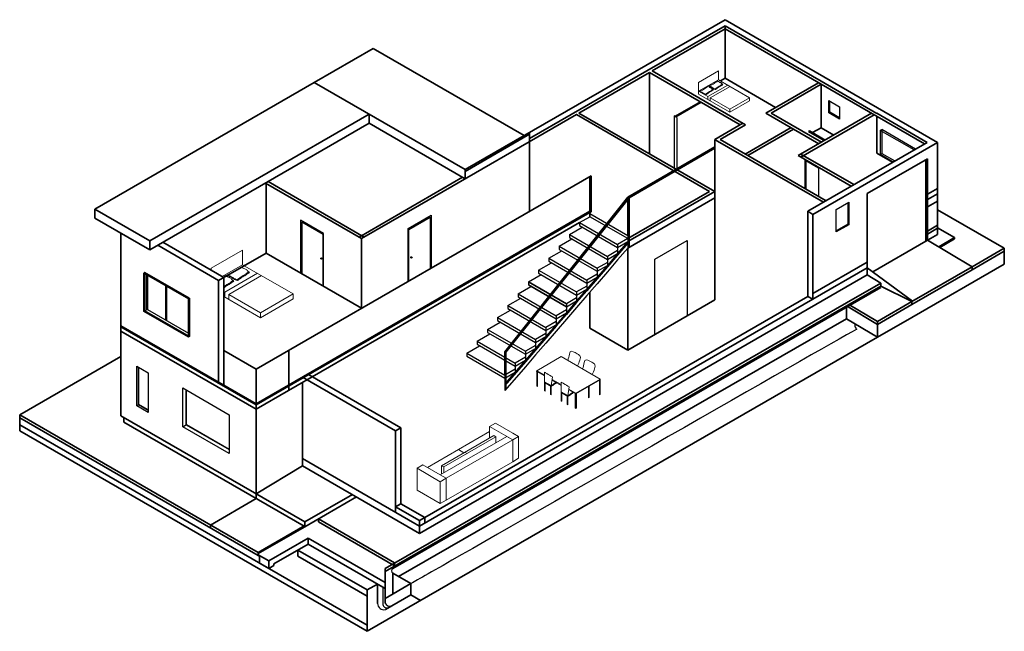
# Model space of a CAD drawing. Units: millimetres. Extents: x -3210 to 34050, y 6347 to 29494.
import ezdxf

# ---------------------------------------------------------------- set-up
doc = ezdxf.new("R2010")
doc.units = ezdxf.units.MM
for name, color, linetype, lineweight in [('A-DOOR', 4, 'Continuous', 25), ('A-FLOR-FIXT', 8, 'Continuous', 18), ('A-FLOR-STRS', 2, 'Continuous', 25), ('A-FURN', 8, 'Continuous', 18), ('A-GLAZ', 3, 'Continuous', 25), ('A-WALL', 7, 'Continuous', 35), ('C-STRM', 5, 'Continuous', 25)]:
    doc.layers.add(name, color=color, linetype=linetype, lineweight=lineweight)

# ---------------------------------------------------------------- blocks, each defined once
blk = doc.blocks.new('stairs')
for p, q in [((17980, 21815), (18368, 22039)), ((19805, 21320), (18368, 22153)), ((19805, 21209), (18368, 22039)), ((17592, 21366), (18076, 21645)), ((17980, 21815), (19417, 20985)), ((17980, 21815), (17980, 21701)), ((17980, 21701), (19417, 20871)), ((17592, 21366), (19029, 20536)), ((17592, 21366), (17592, 21252)), ((17592, 21252), (19029, 20422)), ((19805, 21320), (19805, 20849)), ((17204, 20917), (17688, 21196)), ((17204, 20917), (18641, 20087)), ((17204, 20917), (17204, 20803)), ((19805, 21209), (19417, 20985)), ((19417, 20871), (19805, 21095)), ((19417, 20985), (19417, 20871)), ((19417, 20871), (19417, 20646)), ((16816, 20468), (17300, 20747)), ((17204, 20803), (18641, 19973)), ((19417, 20760), (19029, 20536)), ((19029, 20422), (19417, 20646)), ((19029, 20536), (19029, 20422)), ((16428, 20019), (16912, 20298)), ((16816, 20468), (18253, 19638)), ((16816, 20468), (16816, 20354)), ((16816, 20354), (18253, 19524)), ((19029, 20311), (18641, 20087)), ((18641, 19973), (19029, 20197)), ((19029, 20422), (19029, 20197)), ((16040, 19570), (16524, 19849)), ((16428, 20019), (17865, 19189)), ((16428, 20019), (16428, 19905)), ((16428, 19905), (17865, 19075)), ((18641, 19862), (18253, 19638)), ((18253, 19524), (18641, 19748)), ((18641, 20087), (18641, 19973)), ((18641, 19973), (18641, 19748)), ((15652, 19121), (16136, 19400)), ((16040, 19570), (16040, 19456)), ((18253, 19413), (17865, 19189)), ((18253, 19638), (18253, 19524)), ((18253, 19524), (18253, 19299)), ((15652, 19121), (17089, 18291)), ((15652, 19121), (15652, 19007)), ((15652, 19007), (17089, 18177)), ((17865, 19075), (18253, 19299)), ((17865, 19189), (17865, 19075)), ((17865, 19075), (17865, 18850)), ((15264, 18672), (15748, 18951)), ((15264, 18672), (16701, 17842)), ((15264, 18672), (15264, 18558)), ((17865, 18964), (17477, 18740)), ((17477, 18626), (17865, 18850)), ((17477, 18740), (17477, 18626)), ((14876, 18223), (15360, 18502)), ((15264, 18558), (16701, 17728)), ((17477, 18515), (17089, 18291)), ((17089, 18177), (17477, 18401)), ((17089, 18291), (17089, 18177)), ((17477, 18626), (17477, 18401)), ((14488, 17774), (14972, 18053)), ((14876, 18223), (16314, 17393)), ((14876, 18223), (14876, 18109)), ((14876, 18109), (16314, 17279)), ((17089, 18066), (16701, 17842)), ((16701, 17728), (17089, 17952)), ((17089, 18177), (17089, 17952)), ((14100, 17325), (14584, 17604)), ((14488, 17774), (15926, 16944)), ((14488, 17774), (14488, 17660)), ((14488, 17660), (15926, 16830)), ((16701, 17617), (16314, 17393)), ((16701, 17842), (16701, 17728)), ((16701, 17728), (16701, 17503)), ((13712, 16876), (14196, 17155)), ((14100, 17325), (15538, 16495)), ((14100, 17325), (14100, 17211)), ((14100, 17211), (15538, 16381)), ((16314, 17168), (15926, 16944)), ((16314, 17279), (16701, 17503)), ((16314, 17393), (16314, 17279)), ((16314, 17279), (16314, 17054)), ((13712, 16876), (15150, 16046)), ((13712, 16876), (13712, 16762)), ((15926, 16830), (16314, 17054)), ((15926, 16944), (15926, 16830)), ((15926, 16830), (15926, 16605)), ((13712, 16762), (15150, 15932)), ((15926, 16719), (15538, 16495)), ((15538, 16381), (15926, 16605)), ((15538, 16495), (15538, 16381)), ((15538, 16270), (15150, 16046)), ((15150, 15932), (15538, 16156)), ((15150, 16046), (15150, 15932)), ((15538, 16381), (15538, 16156)), ((15150, 15932), (15150, 15461))]:
    blk.add_line(p, q)
for points in [[(19805, 21095), (19417, 20646), (19029, 20197), (18641, 19748), (18253, 19299), (17865, 18850), (17477, 18401), (17089, 17952), (16701, 17503), (16314, 17054), (15926, 16605), (15150, 15707)], [(19805, 21033), (19417, 20584), (19029, 20135), (18641, 19686), (18253, 19237), (17865, 18788), (17477, 18339), (17089, 17890), (16701, 17441), (16314, 16992), (15926, 16543), (15150, 15645)], [(19805, 20849), (19417, 20400), (19029, 19951), (18641, 19502), (18253, 19053), (17865, 18604), (17477, 18155), (17089, 17706), (16701, 17257), (16314, 16808), (15926, 16359), (15150, 15461)]]:
    blk.add_lwpolyline(points)
blk = doc.blocks.new('dininig')
for p, q in [((17285, 16742), (16365, 16211)), ((18753, 15894), (17285, 16742)), ((16365, 16211), (16646, 16049)), ((16365, 16211), (16365, 15625)), ((16365, 16178), (16646, 16016)), ((16387, 15612), (16387, 16166)), ((16646, 15793), (16646, 15447)), ((16646, 15793), (16900, 15646)), ((16646, 15759), (16900, 15612)), ((16669, 15745), (16669, 15433)), ((16932, 15851), (17281, 15649)), ((16937, 15881), (17281, 15682)), ((17834, 15363), (18753, 15894)), ((17834, 15331), (18753, 15861)), ((18731, 15295), (18731, 15849)), ((18753, 15894), (18753, 15861)), ((18753, 15861), (18753, 15308)), ((16365, 15625), (16387, 15612)), ((16669, 15433), (16646, 15447)), ((16877, 15625), (16877, 15313)), ((16877, 15313), (16900, 15300)), ((16900, 15646), (16900, 15300)), ((17281, 15414), (17281, 15068)), ((17281, 15414), (17536, 15267)), ((17281, 15380), (17536, 15233)), ((17304, 15367), (17304, 15054)), ((17569, 15483), (17834, 15331)), ((17574, 15513), (17834, 15363)), ((17812, 14789), (17812, 15343)), ((17834, 15331), (17834, 14777)), ((17855, 14789), (17855, 15343)), ((18318, 15186), (18318, 15611)), ((18340, 15623), (18340, 15199)), ((18753, 15308), (18731, 15295)), ((17513, 15246), (17513, 14934)), ((17513, 14934), (17536, 14921)), ((17536, 15267), (17536, 14921)), ((18340, 15199), (18318, 15186)), ((17834, 14777), (17812, 14789)), ((17834, 14777), (17855, 14789))]:
    blk.add_line(p, q)
for centre in [(17067, 15749), (17703, 15370)]:
    blk.add_arc(centre, 20.9, 300.0624, 62.4998)
for points, knots in [([(17535, 16602), (17556, 16677), (17584, 16778), (17623, 17007), (17844, 16872), (18083, 16748), (17948, 16515), (17902, 16387), (17901, 16386)], [0, 0, 0, 0, 244.890523, 329.00144, 608.473459, 721.036072, 1125.699972, 1130.16971, 1130.16971, 1130.16971, 1130.16971]), ([(18091, 16281), (18113, 16356), (18141, 16457), (18180, 16685), (18401, 16551), (18639, 16427), (18505, 16193), (18458, 16066), (18458, 16064)], [0, 0, 0, 0, 244.890523, 329.00144, 608.473459, 721.036072, 1125.699972, 1130.16971, 1130.16971, 1130.16971, 1130.16971]), ([(16646, 16154), (16676, 16136), (16778, 16077), (16880, 16018), (16952, 15977)], [0, 0, 0, 0, 105.813735, 353.485059, 353.485059, 353.485059, 353.485059]), ([(16900, 15612), (16921, 15626), (16983, 15668), (17044, 15709), (17078, 15731)], [0, 0, 0, 0, 75.861008, 223.095154, 223.095154, 223.095154, 223.095154]), ([(17281, 15775), (17312, 15757), (17414, 15698), (17516, 15639), (17587, 15598)], [0, 0, 0, 0, 105.813735, 353.485059, 353.485059, 353.485059, 353.485059]), ([(17536, 15233), (17557, 15247), (17618, 15289), (17680, 15330), (17713, 15352)], [0, 0, 0, 0, 75.861008, 223.095154, 223.095154, 223.095154, 223.095154])]:
    blk.add_open_spline(points, degree=3, knots=knots)
for points in [[(16646, 15793), (16646, 15913), (16646, 16033), (16646, 16154)], [(16900, 15646), (16917, 15756), (16934, 15867), (16952, 15977)], [(16900, 15646), (16959, 15686), (17018, 15727), (17077, 15767)], [(17281, 15414), (17281, 15534), (17281, 15655), (17281, 15775)], [(17536, 15267), (17553, 15377), (17570, 15488), (17587, 15598)], [(17536, 15267), (17595, 15308), (17654, 15348), (17713, 15389)]]:
    blk.add_open_spline(points, degree=3)
blk = doc.blocks.new('sofa')
for p, q in [((14566, 14099), (14789, 14228)), ((14789, 14228), (15446, 13849)), ((12217, 12549), (14566, 13905)), ((15446, 13591), (14566, 14099)), ((14566, 14099), (14566, 13658)), ((15669, 13720), (15446, 13849)), ((12705, 12267), (15222, 13720)), ((12758, 12614), (14730, 13753)), ((12838, 12568), (14810, 13706)), ((12929, 12138), (15446, 13591)), ((14730, 13753), (14810, 13706)), ((14810, 13706), (14810, 13482)), ((15222, 13720), (15446, 13591)), ((15669, 13720), (15446, 13591)), ((15446, 13591), (15446, 12765)), ((15446, 12765), (15446, 13591)), ((15669, 12894), (15669, 13720)), ((13391, 13227), (13601, 13101)), ((13637, 13122), (13717, 13076)), ((12929, 11312), (15446, 12765)), ((15669, 12894), (15446, 12765)), ((11825, 12517), (12049, 12646)), ((12705, 12009), (11825, 12517)), ((11825, 12517), (11825, 11691)), ((12049, 12646), (12705, 12267)), ((12758, 12297), (12758, 12614)), ((12758, 12614), (12838, 12568)), ((12838, 12343), (12838, 12568)), ((12929, 12138), (12705, 12267)), ((12929, 12138), (12705, 12009)), ((12705, 11183), (12705, 12009)), ((12929, 11312), (12929, 12138)), ((12705, 11183), (11825, 11691)), ((12929, 11312), (12705, 11183))]:
    blk.add_line(p, q)
blk = doc.blocks.new('DOOR-900')
for p, q in [((0, 2000), (866, 2500)), ((17, 1960), (823, 2425)), ((823, 2425), (823, 475)), ((866, 2500), (866, 500)), ((0, 0), (0, 2000)), ((17, 10), (17, 1960))]:
    blk.add_line(p, q)
blk = doc.blocks.new('SINK-BOWL')
for p, q in [((0, 134), (4, 114)), ((503, 200), (507, 180))]:
    blk.add_line(p, q)
blk.add_arc((252, 15), 27.2, 169.8269, 214.4645)
for points, knots in [([(0, 134), (17, 144), (48, 164), (141, 193), (223, 262), (299, 304), (323, 317)], [0, 0, 0, 0, 58.087892, 110.763148, 288.499212, 372.227316, 372.227316, 372.227316, 372.227316]), ([(0, 134), (35, 118), (95, 90), (165, 42), (208, 26), (225, 20)], [0, 0, 0, 0, 115.602535, 198.179559, 253.050311, 253.050311, 253.050311, 253.050311]), ([(4, 114), (39, 98), (99, 70), (169, 21), (212, 6), (230, 0)], [0, 0, 0, 0, 115.602535, 198.179559, 253.050311, 253.050311, 253.050311, 253.050311]), ([(225, 20), (250, 38), (298, 73), (355, 118), (422, 143), (427, 163), (474, 187), (475, 189), (476, 191), (485, 194), (494, 197), (503, 200)], [0, 0, 0, 0, 88.806256, 177.702848, 228.702299, 271.942722, 280.573254, 305.589533, 305.589533, 305.589533, 331.140258, 331.140258, 331.140258, 331.140258]), ([(230, 0), (254, 17), (303, 52), (359, 98), (426, 123), (432, 143), (478, 167), (479, 169), (480, 171), (489, 174), (498, 177), (507, 180)], [0, 0, 0, 0, 88.806256, 177.702848, 228.702299, 271.942722, 280.573254, 305.589533, 305.589533, 305.589533, 331.140258, 331.140258, 331.140258, 331.140258]), ([(323, 317), (342, 304), (373, 283), (415, 265), (451, 255), (460, 225), (476, 216), (483, 212), (490, 208), (496, 204), (503, 200)], [0, 0, 0, 0, 68.223474, 110.975196, 140.481146, 170.504076, 194.596577, 194.596577, 194.596577, 217.431117, 217.431117, 217.431117, 217.431117])]:
    blk.add_open_spline(points, degree=3, knots=knots)

msp = doc.modelspace()

# ---------------------------------------------------------------- linework, layer by layer
at = {"layer": 'A-DOOR'}
for p, q in [((21551, 25852), (21551, 23884)), ((21653, 25793), (21551, 25852)), ((21653, 25793), (21653, 23825)), ((26501, 24208), (26501, 23108)), ((26540, 24166), (27012, 23893)), ((26540, 24166), (26540, 23086)), ((27012, 23893), (27012, 22813)), ((27020, 23908), (27020, 22808)), ((20824, 20429), (22052, 21138)), ((22052, 21138), (22052, 18287)), ((20824, 17578), (20824, 20429))]:
    msp.add_line(p, q, dxfattribs=at)
for centre, radius in [((11613, 20495), 26.5), ((8205, 20457), 23.3)]:
    msp.add_circle(centre, radius, dxfattribs=at)
at = {"layer": 'A-FLOR-FIXT'}
for p, q in [((22477, 27122), (23234, 27559)), ((22477, 26786), (23234, 27222)), ((23234, 27222), (23234, 27559)), ((23234, 27222), (24413, 26542)), ((22477, 26786), (22477, 27122)), ((22825, 26585), (23582, 27022)), ((22918, 26531), (23674, 26968)), ((22477, 26786), (22477, 26670)), ((22825, 26585), (22477, 26786)), ((23657, 25990), (22477, 26670)), ((22825, 26585), (22825, 26470)), ((23657, 26105), (22918, 26531)), ((22918, 26531), (22918, 26416)), ((24413, 26542), (23657, 26105)), ((24413, 26542), (24413, 26426)), ((24413, 26426), (23657, 25990)), ((23657, 26105), (23657, 25990)), ((4040, 20090), (5219, 20770)), ((5219, 20223), (5219, 20770)), ((4448, 19778), (5219, 20223)), ((5219, 20223), (7139, 19115)), ((4040, 20013), (4040, 20090)), ((4553, 19186), (5785, 19897)), ((4654, 19838), (4661, 19805)), ((4705, 19098), (5936, 19809)), ((5473, 19945), (5480, 19912)), ((4882, 19617), (4889, 19584)), ((4553, 19186), (4515, 19208)), ((5907, 18217), (4515, 19021)), ((4553, 19186), (4553, 18998)), ((5907, 18404), (4705, 19098)), ((4705, 19098), (4705, 18911)), ((7139, 19115), (5907, 18404)), ((7139, 19115), (7139, 18928)), ((7139, 18928), (5907, 18217)), ((5907, 18404), (5907, 18217))]:
    msp.add_line(p, q, dxfattribs=at)
msp.add_arc((5064, 19645), 44.3, 169.8269, 214.4645, dxfattribs=at)
for points, knots in [([(4654, 19838), (4681, 19855), (4733, 19886), (4883, 19933), (5016, 20046), (5141, 20114), (5180, 20136)], [0, 0, 0, 0, 94.538199, 180.267318, 469.533235, 605.800947, 605.800947, 605.800947, 605.800947]), ([(5180, 20136), (5211, 20114), (5261, 20079), (5330, 20051), (5387, 20034), (5402, 19986), (5428, 19971), (5440, 19964), (5451, 19958), (5462, 19951), (5473, 19945)], [0, 0, 0, 0, 68.223474, 110.975196, 140.481146, 170.504076, 194.596577, 194.596577, 194.596577, 217.431117, 217.431117, 217.431117, 217.431117]), ([(4590, 19808), (4620, 19786), (4670, 19751), (4739, 19723), (4797, 19706), (4811, 19658), (4837, 19643), (4849, 19636), (4860, 19630), (4871, 19623), (4882, 19617)], [0, 0, 0, 0, 68.223474, 110.975196, 140.481146, 170.504076, 194.596577, 194.596577, 194.596577, 217.431117, 217.431117, 217.431117, 217.431117]), ([(4654, 19838), (4711, 19812), (4809, 19767), (4922, 19687), (4993, 19662), (5021, 19652)], [0, 0, 0, 0, 188.143434, 322.53776, 411.840053, 411.840053, 411.840053, 411.840053]), ([(4661, 19805), (4718, 19779), (4816, 19734), (4929, 19654), (5000, 19629), (5028, 19619)], [0, 0, 0, 0, 188.143434, 322.53776, 411.840053, 411.840053, 411.840053, 411.840053]), ([(5021, 19652), (5060, 19681), (5139, 19738), (5231, 19812), (5341, 19853), (5349, 19884), (5425, 19923), (5427, 19927), (5429, 19930), (5443, 19935), (5458, 19940), (5473, 19945)], [0, 0, 0, 0, 88.806256, 177.702848, 228.702299, 271.942722, 280.573254, 305.589533, 305.589533, 305.589533, 331.140258, 331.140258, 331.140258, 331.140258]), ([(5028, 19619), (5067, 19648), (5146, 19705), (5238, 19779), (5348, 19820), (5357, 19852), (5432, 19891), (5434, 19894), (5436, 19897), (5451, 19902), (5465, 19907), (5480, 19912)], [0, 0, 0, 0, 88.806256, 177.702848, 228.702299, 271.942722, 280.573254, 305.589533, 305.589533, 305.589533, 331.140258, 331.140258, 331.140258, 331.140258]), ([(4515, 19386), (4525, 19394), (4574, 19430), (4641, 19483), (4750, 19525), (4759, 19556), (4835, 19595), (4837, 19599), (4838, 19602), (4853, 19607), (4867, 19612), (4882, 19617)], [63.928623, 63.928623, 63.928623, 63.928623, 88.806256, 177.702848, 228.702299, 271.942722, 280.573254, 305.589533, 305.589533, 305.589533, 331.140258, 331.140258, 331.140258, 331.140258]), ([(4515, 19348), (4528, 19357), (4579, 19396), (4648, 19451), (4757, 19492), (4766, 19523), (4842, 19562), (4844, 19566), (4845, 19569), (4860, 19574), (4874, 19579), (4889, 19584)], [58.503558, 58.503558, 58.503558, 58.503558, 88.806256, 177.702848, 228.702299, 271.942722, 280.573254, 305.589533, 305.589533, 305.589533, 331.140258, 331.140258, 331.140258, 331.140258])]:
    msp.add_open_spline(points, degree=3, knots=knots, dxfattribs=at)
msp.add_open_spline([(4492, 19752), (4524, 19772), (4557, 19790), (4590, 19808)], degree=3, dxfattribs=at)
at = {"layer": 'A-GLAZ'}
for p, q in [((27408, 25967), (27408, 26432)), ((27408, 26432), (27810, 26200)), ((27449, 25991), (27449, 26408)), ((27810, 26200), (27810, 25735)), ((27408, 25967), (27450, 25992)), ((27810, 25735), (27408, 25967)), ((27810, 25784), (27449, 25992)), ((29351, 25299), (29414, 25335)), ((29351, 25299), (29351, 24399)), ((30634, 24566), (29358, 25303)), ((29414, 25335), (29414, 24435)), ((30690, 24598), (29414, 25335)), ((29351, 24399), (29414, 24435)), ((29351, 24399), (29848, 24112)), ((29414, 24435), (29910, 24148)), ((27692, 22310), (28168, 22585)), ((28133, 22565), (28133, 21755)), ((28168, 22585), (28168, 21735)), ((27692, 21460), (27692, 22310)), ((28133, 21755), (27692, 21500)), ((28168, 21735), (27692, 21460)), ((28133, 21755), (28168, 21735)), ((1527, 19928), (1484, 19903)), ((1484, 18453), (1484, 19903)), ((1484, 19903), (3172, 18928)), ((1527, 18478), (1527, 19928)), ((3216, 18953), (1527, 19928)), ((1573, 19852), (1573, 18504)), ((1620, 19824), (1620, 18532)), ((2311, 19426), (2311, 18134)), ((2345, 19406), (2345, 18114)), ((3172, 18928), (3216, 18953)), ((3172, 17478), (3172, 18928)), ((3216, 18953), (3216, 17503)), ((1620, 18532), (1484, 18453)), ((3172, 17478), (1484, 18453)), ((3216, 17503), (1527, 18478)), ((1620, 18532), (3172, 17636)), ((3216, 17503), (3172, 17478)), ((1218, 14881), (1218, 16381)), ((1218, 16381), (1651, 16131)), ((1284, 14920), (1284, 16343)), ((1301, 14930), (1301, 16333)), ((1651, 16131), (1651, 14631)), ((2957, 15557), (4717, 14541)), ((2957, 14089), (2957, 15557)), ((3086, 14163), (3086, 15482)), ((3104, 14173), (3104, 15472)), ((1218, 14881), (1301, 14931)), ((1651, 14709), (1284, 14920)), ((1651, 14729), (1301, 14930)), ((1651, 14631), (1218, 14881)), ((4717, 14541), (4717, 13072)), ((2957, 14089), (3104, 14173)), ((3086, 14163), (4717, 13222)), ((3104, 14173), (4717, 13242)), ((4717, 13072), (2957, 14089))]:
    msp.add_line(p, q, dxfattribs=at)
at = {"layer": 'A-WALL'}
for p, q in [((23482, 29494), (13651, 23819)), ((31524, 24851), (23482, 29494)), ((23482, 29266), (20525, 27559)), ((23482, 29151), (20723, 27559)), ((27121, 27165), (23482, 29266)), ((23482, 29266), (23482, 27278)), ((27119, 27051), (23482, 29151)), ((10169, 28409), (7935, 27119)), ((15885, 25109), (10169, 28409)), ((20525, 27559), (17654, 25901)), ((20624, 27501), (17955, 25960)), ((24059, 25518), (20624, 27501)), ((20624, 27501), (20624, 24419)), ((24260, 25517), (20723, 27559)), ((23482, 27278), (23310, 27178)), ((23482, 27278), (25397, 26172)), ((7935, 27119), (-364, 22327)), ((13651, 23819), (7935, 27119)), ((27020, 27109), (25028, 25959)), ((27119, 27051), (25226, 25958)), ((31029, 24794), (27119, 27051)), ((27119, 27051), (27119, 25407)), ((29224, 25950), (27121, 27165)), ((22550, 26389), (21585, 25832)), ((22584, 26369), (21619, 25812)), ((1715, 21127), (10014, 25919)), ((10014, 25576), (10014, 25919)), ((17856, 25903), (11919, 22476)), ((17654, 25901), (16083, 24994)), ((17856, 25903), (17852, 25901)), ((22896, 22993), (17856, 25903)), ((23094, 22993), (17955, 25960)), ((27033, 24801), (25028, 25959)), ((27132, 24858), (25226, 25958)), ((29026, 25952), (26253, 24351)), ((29123, 25894), (26352, 24294)), ((31128, 24851), (29222, 25951)), ((29224, 25836), (29224, 24439)), ((1715, 20784), (10014, 25576)), ((13651, 23476), (10014, 25576)), ((24158, 25575), (23094, 24961)), ((24260, 25517), (23295, 24959)), ((25979, 25409), (24247, 24409)), ((26078, 25352), (24346, 24352)), ((26789, 25221), (27119, 25407)), ((27119, 25407), (27601, 25129)), ((13651, 23754), (16083, 25158)), ((15885, 25109), (13651, 23819)), ((16083, 24880), (16083, 25223)), ((26641, 25258), (26684, 25282)), ((27232, 24917), (26641, 25258)), ((27275, 24941), (26684, 25282)), ((16083, 24880), (16083, 22242)), ((19805, 22781), (23094, 24679)), ((19851, 22757), (23094, 24629)), ((23196, 24902), (23094, 24961)), ((23094, 24961), (23094, 22748)), ((27206, 22587), (23196, 24902)), ((27305, 22644), (23295, 24959)), ((31128, 24851), (26618, 22247)), ((31524, 24851), (26799, 22123)), ((31524, 21371), (31524, 24851)), ((28257, 23194), (26253, 24351)), ((28356, 23251), (26352, 24408)), ((31143, 24231), (28861, 22914)), ((29819, 24096), (29224, 24439)), ((31143, 21151), (31143, 24231)), ((31079, 21115), (31079, 24195)), ((31099, 21126), (31099, 24206)), ((18411, 23586), (5742, 16271)), ((9630, 21268), (13552, 23533)), ((13651, 23476), (13651, 23819)), ((18368, 22243), (18368, 23561)), ((18411, 22228), (18411, 23586)), ((9729, 21211), (6092, 23311)), ((6112, 23323), (6112, 20662)), ((9828, 21268), (6191, 23368)), ((31524, 23111), (31079, 22855)), ((19805, 22781), (15150, 16930)), ((15183, 16911), (19851, 22757)), ((23094, 22993), (19805, 21095)), ((22896, 22993), (19805, 21209)), ((19805, 21320), (19805, 22781)), ((19805, 22781), (19851, 22757)), ((19805, 20849), (23094, 22748)), ((19851, 22757), (19852, 20876)), ((23094, 22748), (23094, 18889)), ((28861, 22914), (28861, 19834)), ((31524, 22902), (31079, 22646)), ((9729, 21211), (11919, 22476)), ((31524, 22627), (31079, 22370)), ((-364, 22327), (1715, 21127)), ((-364, 22327), (-364, 21985)), ((1715, 20784), (-364, 21985)), ((18368, 22243), (5742, 14953)), ((18368, 22203), (5742, 14913)), ((18368, 22203), (18411, 22228)), ((18368, 22153), (18368, 22203)), ((18368, 22039), (18368, 22153)), ((18411, 22228), (18411, 22268)), ((26618, 22247), (26618, 19023)), ((26618, 22247), (26799, 22123)), ((26799, 22123), (26799, 18918)), ((34050, 20845), (31524, 22303)), ((17980, 21815), (5742, 14749)), ((31524, 21714), (31143, 21494)), ((32167, 21246), (31524, 21618)), ((619, 21417), (619, 17707)), ((31524, 21371), (31079, 21115)), ((31524, 21600), (31143, 21380)), ((31566, 20899), (32167, 21246)), ((32167, 21246), (32167, 21196)), ((1715, 21127), (1715, 20784)), ((4317, 19625), (2012, 20956)), ((2012, 20956), (4317, 19625)), ((2210, 21070), (4515, 19739)), ((9729, 21211), (9729, 18573)), ((31079, 21115), (29070, 19954)), ((31079, 21115), (29070, 19954)), ((31079, 21115), (29070, 19954)), ((31143, 21151), (32831, 20141)), ((31609, 20874), (32167, 21196)), ((6112, 20662), (4317, 19625)), ((9729, 18573), (6112, 20662)), ((19805, 20849), (19805, 16990)), ((32831, 20141), (34050, 20845)), ((32831, 20027), (34050, 20730)), ((34050, 20845), (34050, 20730)), ((34050, 20730), (34050, 20245)), ((28861, 20318), (26799, 19128)), ((30550, 18224), (34050, 20245)), ((30550, 18824), (32831, 20141)), ((32831, 20141), (32831, 20027)), ((28861, 19834), (11921, 10054)), ((28861, 20109), (26799, 18918)), ((28861, 20109), (30576, 18839)), ((28861, 19834), (29371, 19529)), ((30550, 18710), (32831, 20027)), ((4317, 19625), (4317, 15736)), ((4515, 19739), (4515, 15622)), ((10626, 8616), (29371, 19414)), ((16040, 19570), (17477, 18740)), ((16040, 19456), (17477, 18626)), ((29371, 19529), (28072, 18779)), ((29371, 19529), (29371, 19414)), ((29371, 19414), (30550, 18824)), ((10911, 8721), (29371, 19355)), ((26618, 19023), (12117, 10651)), ((18368, 19186), (18368, 17820)), ((26618, 19023), (26799, 18918)), ((28072, 18779), (10626, 8730)), ((26799, 18918), (11921, 10329)), ((19805, 16990), (23094, 18889)), ((28072, 18664), (28072, 18179)), ((28072, 18664), (29251, 17960)), ((28169, 18720), (29251, 18074)), ((29251, 18074), (30550, 18824)), ((29251, 17960), (30550, 18710)), ((30550, 18824), (30550, 18710)), ((5742, 14953), (619, 17911)), ((11130, 8421), (28072, 18179)), ((28072, 18179), (29251, 17474)), ((29251, 17474), (30550, 18224)), ((29251, 17474), (29251, 18074)), ((5742, 14913), (619, 17871)), ((5742, 14749), (619, 17707)), ((619, 17707), (619, 14507)), ((19805, 16990), (18368, 17820)), ((29251, 17474), (9937, 6347)), ((5742, 16271), (4515, 16980)), ((6969, 16980), (6969, 15458)), ((15150, 16046), (15150, 16930)), ((15183, 15499), (15183, 16911)), ((-3210, 14538), (619, 16748)), ((5742, 16271), (5742, 14749)), ((11207, 14052), (7694, 16080)), ((16365, 16211), (16365, 16178)), ((7497, 15967), (11010, 13938)), ((7497, 15763), (7497, 12608)), ((17304, 15054), (17281, 15068)), ((-3210, 14538), (-3210, 13938)), ((5817, 9326), (-3210, 14538)), ((5742, 14749), (5742, 11550)), ((5817, 9211), (-3210, 14423)), ((9937, 6576), (-3210, 14166)), ((7586, 10485), (619, 14507)), ((732, 14442), (732, 14264)), ((7551, 10327), (732, 14264)), ((9937, 6347), (-3210, 13938)), ((11010, 13938), (11207, 14052)), ((11010, 10854), (11010, 13938)), ((11207, 11177), (11207, 14052)), ((11740, 10433), (7497, 12883)), ((7497, 12608), (5742, 11550)), ((11921, 10054), (7497, 12608)), ((5742, 11372), (4008, 10370)), ((5742, 11550), (5742, 11372)), ((9380, 11521), (7586, 10485)), ((7586, 10307), (9534, 11432)), ((11010, 11063), (11207, 11177)), ((11010, 11063), (11921, 10538)), ((11207, 11177), (12117, 10651)), ((7586, 10485), (7586, 10307)), ((10978, 8933), (8092, 10599)), ((8092, 10599), (8092, 10485)), ((10978, 8819), (8092, 10485)), ((11921, 10329), (11740, 10433)), ((12117, 10651), (11921, 10538)), ((11921, 10538), (11921, 10054)), ((12117, 10651), (12117, 10442)), ((4008, 10370), (4008, 10256)), ((7586, 10347), (5817, 9326)), ((7586, 10307), (5817, 9286)), ((6215, 9013), (7711, 9877)), ((10626, 8194), (7711, 9877)), ((7711, 9877), (7711, 9648)), ((5817, 9326), (5817, 9211)), ((6413, 8899), (7711, 9648)), ((9937, 7911), (7319, 9422)), ((7319, 9422), (7319, 9193)), ((10626, 7966), (7711, 9648)), ((5817, 9243), (6215, 9013)), ((5817, 9211), (5860, 9186)), ((5860, 9186), (5860, 8929)), ((6215, 8725), (6215, 9013)), ((9937, 7682), (7319, 9193)), ((5860, 8929), (6215, 8725)), ((6215, 8725), (6413, 8839)), ((6413, 8839), (6413, 8899)), ((10626, 8730), (10626, 8130)), ((10978, 8933), (10978, 8819)), ((10911, 8548), (11593, 8154)), ((10911, 8548), (10911, 7760)), ((10329, 8137), (9937, 7911)), ((9937, 7911), (9937, 6347)), ((10329, 8137), (10329, 7395)), ((11593, 8154), (10626, 7595)), ((10626, 8130), (10626, 7417)), ((11593, 8154), (11593, 7726)), ((11593, 7726), (10628, 7169)), ((11593, 7726), (11959, 7515))]:
    msp.add_line(p, q, dxfattribs=at)
at = {"layer": 'C-STRM'}
msp.add_line((10527, 8023), (10527, 7359), dxfattribs=at)
for centre, radius, start, end in [((10961, 8634), 100, 120, 240), ((10583, 7420), 255, 185.6116, 280.2153), ((10693, 7406), 173, 195.7516, 296.7805), ((10804, 7484), 190, 200.5452, 286.9044)]:
    msp.add_arc(centre, radius, start, end, dxfattribs=at)
for points, knots in [([(28386, 17991), (28390, 17928), (28396, 17845), (28454, 17793), (28468, 17781)], [0, 0, 0, 0, 178.181356, 231.903074, 231.903074, 231.903074, 231.903074]), ([(28468, 17781), (26927, 16930), (14815, 9982), (11946, 8349), (11672, 8196), (11593, 8154)], [0, 0, 0, 0, 5280.088451, 5953.3657, 6221.129999, 6221.129999, 6221.129999, 6221.129999])]:
    msp.add_open_spline(points, degree=3, knots=knots, dxfattribs=at)

# ---------------------------------------------------------------- block references
at = {"layer": 'A-DOOR'}
msp.add_blockref('DOOR-900', (11495, 19593), dxfattribs=at)
at = {"layer": 'A-DOOR', "extrusion": (0, 0, -1), "zscale": -1}
msp.add_blockref('DOOR-900', (-8287, 19406), dxfattribs=at)
at = {"layer": 'A-FLOR-FIXT'}
for p in [(22524, 26650), (22887, 26851)]:
    msp.add_blockref('SINK-BOWL', p, dxfattribs=at)
at = {"layer": 'A-FLOR-STRS'}
msp.add_blockref('stairs', (0, 0), dxfattribs=at)
at = {"layer": 'A-FURN'}
for name in ['dininig', 'sofa']:
    msp.add_blockref(name, (0, 0), dxfattribs=at)

doc.saveas('drawing.dxf')
